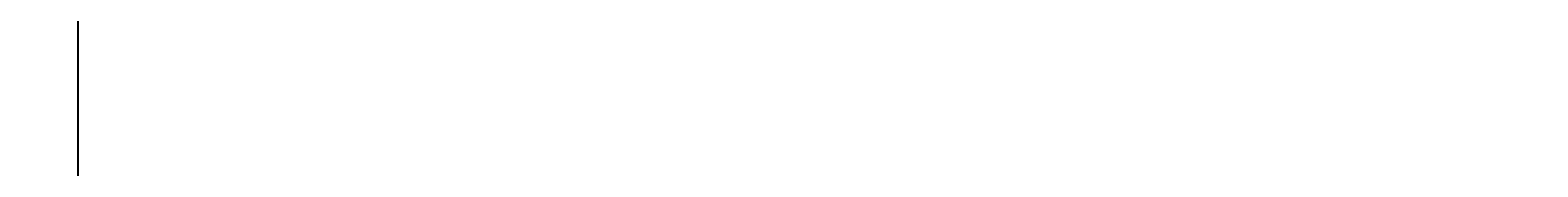
# Model space of a CAD drawing. Units: inches. Extents: x 35362 to 73946, y 43607 to 67532.
# Tile 103 of 134: x 50119 to 50761, y 49328 to 49386. Entities that reach past the tile are written whole.
import ezdxf

# ---------------------------------------------------------------- set-up
doc = ezdxf.new("R2010")
doc.units = ezdxf.units.IN
doc.header["$MEASUREMENT"] = 0
doc.layers.add('A-ANNO-DIMS', color=2, linetype='Continuous', lineweight=18)
doc.styles.get("Standard").update_dxf_attribs({"font": 'arial.ttf'})
doc.dimstyles.get("Standard").update_dxf_attribs({"dimtxt": 0.18, "dimasz": 0.18, "dimexe": 0.18, "dimexo": 0.0625, "dimgap": 0.09, "dimtad": 0, "dimtih": 1, "dimtoh": 1, "dimdec": 4, "dimzin": 0, "dimdsep": 46, "dimtxsty": 'Standard', "dimcen": 0.09, "dimadec": 0, "dimazin": 0, "dimtfac": 1, "dimtdec": 4, "dimtofl": 0, "dimtmove": 0, "dimatfit": 3, "dimfxl": 1, "dimtolj": 1, "dimtzin": 0, "dimarcsym": 0})

# ---------------------------------------------------------------- blocks, each defined once
blk = doc.blocks.new('*D11')
at = {"layer": 'A-ANNO-DIMS', "color": 0, "lineweight": -2, "transparency": 16777216}
for p, q in [((47978.66, 56028.77), (47978.66, 43606.68)), ((53109.76, 56028.77), (53109.76, 43606.68)), ((47978.84, 43606.86), (50543.87, 43606.86)), ((53109.58, 43606.86), (50544.55, 43606.86))]:
    blk.add_line(p, q, dxfattribs=at)
at = {"layer": 'A-ANNO-DIMS', "color": 0, "transparency": 16777216}
for points in [[(47978.84, 43606.89), (47978.84, 43606.83), (47978.66, 43606.86)], [(53109.58, 43606.89), (53109.58, 43606.83), (53109.76, 43606.86)]]:
    blk.add_solid(points, dxfattribs=at)
at = {"layer": 'Defpoints', "color": 0, "transparency": 16777216}
for p in [(47978.66, 56028.84), (53109.76, 56028.84), (53109.76, 43606.86)]:
    blk.add_point(p, dxfattribs=at)
at = {"layer": 'A-ANNO-DIMS', "color": 0, "transparency": 16777216, "insert": (50544.21, 43606.86), "char_height": 0.18, "attachment_point": 5}
blk.add_mtext('\\A1;5131', dxfattribs=at)
blk = doc.blocks.new('*D13')
at = {"layer": 'A-ANNO-DIMS', "color": 0, "lineweight": -2, "transparency": 16777216}
for p, q in [((48373.49, 51694.02), (48373.49, 43606.68)), ((51029.04, 51694.02), (51029.04, 43606.68)), ((48373.67, 43606.86), (49700.8, 43606.86)), ((51028.86, 43606.86), (49701.73, 43606.86))]:
    blk.add_line(p, q, dxfattribs=at)
at = {"layer": 'A-ANNO-DIMS', "color": 0, "transparency": 16777216}
for points in [[(48373.67, 43606.89), (48373.67, 43606.83), (48373.49, 43606.86)], [(51028.86, 43606.89), (51028.86, 43606.83), (51029.04, 43606.86)]]:
    blk.add_solid(points, dxfattribs=at)
at = {"layer": 'Defpoints', "color": 0, "transparency": 16777216}
for p in [(48373.49, 51694.09), (51029.04, 51694.09), (51029.04, 43606.86)]:
    blk.add_point(p, dxfattribs=at)
at = {"layer": 'A-ANNO-DIMS', "color": 0, "transparency": 16777216, "insert": (49701.27, 43606.86), "char_height": 0.18, "attachment_point": 5}
blk.add_mtext('\\A1;2655.6', dxfattribs=at)
blk = doc.blocks.new('*D17')
at = {"layer": 'A-ANNO-DIMS', "color": 0, "lineweight": -2, "transparency": 16777216}
for p, q in [((49923.31, 61293.22), (49923.31, 43606.68)), ((51913.93, 61293.22), (51913.93, 43606.68)), ((49923.49, 43606.86), (50918.16, 43606.86)), ((51913.75, 43606.86), (50919.07, 43606.86))]:
    blk.add_line(p, q, dxfattribs=at)
at = {"layer": 'A-ANNO-DIMS', "color": 0, "transparency": 16777216}
for points in [[(49923.49, 43606.89), (49923.49, 43606.83), (49923.31, 43606.86)], [(51913.75, 43606.89), (51913.75, 43606.83), (51913.93, 43606.86)]]:
    blk.add_solid(points, dxfattribs=at)
at = {"layer": 'Defpoints', "color": 0, "transparency": 16777216}
for p in [(49923.31, 61293.29), (51913.93, 61293.29), (51913.93, 43606.86)]:
    blk.add_point(p, dxfattribs=at)
at = {"layer": 'A-ANNO-DIMS', "color": 0, "transparency": 16777216, "insert": (50918.62, 43606.86), "char_height": 0.18, "attachment_point": 5}
blk.add_mtext('\\A1;1990.6', dxfattribs=at)
blk = doc.blocks.new('*D40')
at = {"layer": 'A-ANNO-DIMS', "color": 0, "lineweight": -2, "transparency": 16777216}
for p, q in [((56873.54, 53351.53), (35361.77, 53351.53)), ((35361.95, 53351.35), (35361.95, 51333.28)), ((35361.95, 49314.85), (35361.95, 51332.92)), ((51806.45, 49314.67), (35361.77, 49314.67))]:
    blk.add_line(p, q, dxfattribs=at)
at = {"layer": 'A-ANNO-DIMS', "color": 0, "transparency": 16777216}
for points in [[(35361.92, 53351.35), (35361.98, 53351.35), (35361.95, 53351.53)], [(35361.92, 49314.85), (35361.98, 49314.85), (35361.95, 49314.67)]]:
    blk.add_solid(points, dxfattribs=at)
at = {"layer": 'Defpoints', "color": 0, "transparency": 16777216}
for p in [(35361.95, 53351.53), (56873.6, 53351.53), (51806.52, 49314.67)]:
    blk.add_point(p, dxfattribs=at)
at = {"layer": 'A-ANNO-DIMS', "color": 0, "transparency": 16777216, "insert": (35361.95, 51333.1), "char_height": 0.18, "attachment_point": 5}
blk.add_mtext('\\A1;4036.9', dxfattribs=at)
blk = doc.blocks.new('*D67')
at = {"layer": 'A-ANNO-DIMS', "color": 0, "lineweight": -2, "transparency": 16777216}
for p, q in [((56873.54, 53351.53), (35361.77, 53351.53)), ((35361.95, 53351.35), (35361.95, 49400.89)), ((35361.95, 45450.07), (35361.95, 49400.53)), ((53793.58, 45449.89), (35361.77, 45449.89))]:
    blk.add_line(p, q, dxfattribs=at)
at = {"layer": 'A-ANNO-DIMS', "color": 0, "transparency": 16777216}
for points in [[(35361.92, 53351.35), (35361.98, 53351.35), (35361.95, 53351.53)], [(35361.92, 45450.07), (35361.98, 45450.07), (35361.95, 45449.89)]]:
    blk.add_solid(points, dxfattribs=at)
at = {"layer": 'Defpoints', "color": 0, "transparency": 16777216}
for p in [(35361.95, 53351.53), (56873.6, 53351.53), (53793.64, 45449.89)]:
    blk.add_point(p, dxfattribs=at)
at = {"layer": 'A-ANNO-DIMS', "color": 0, "transparency": 16777216, "insert": (35361.95, 49400.71), "char_height": 0.18, "attachment_point": 5}
blk.add_mtext('\\A1;7901.6', dxfattribs=at)
blk = doc.blocks.new('*D107')
at = {"layer": 'A-ANNO-DIMS', "color": 0, "lineweight": -2, "transparency": 16777216}
for p, q in [((50139.56, 59850.01), (50139.56, 43606.68)), ((51320.81, 59850.01), (51320.81, 43606.68)), ((50139.74, 43606.86), (50729.73, 43606.86)), ((51320.63, 43606.86), (50730.64, 43606.86))]:
    blk.add_line(p, q, dxfattribs=at)
at = {"layer": 'A-ANNO-DIMS', "color": 0, "transparency": 16777216}
for points in [[(50139.74, 43606.89), (50139.74, 43606.83), (50139.56, 43606.86)], [(51320.63, 43606.89), (51320.63, 43606.83), (51320.81, 43606.86)]]:
    blk.add_solid(points, dxfattribs=at)
at = {"layer": 'Defpoints', "color": 0, "transparency": 16777216}
for p in [(50139.56, 59850.08), (51320.81, 59850.08), (51320.81, 43606.86)]:
    blk.add_point(p, dxfattribs=at)
at = {"layer": 'A-ANNO-DIMS', "color": 0, "transparency": 16777216, "insert": (50730.19, 43606.86), "char_height": 0.18, "attachment_point": 5}
blk.add_mtext('\\A1;1181.3', dxfattribs=at)

msp = doc.modelspace()

# ---------------------------------------------------------------- dimensions: what is measured, and where the dimension line sits
at = {"layer": 'A-ANNO-DIMS'}
for base, p1, p2, override, picture, middle in [((51913.931, 43606.859), (49923.307, 61293.286), (51913.931, 61293.286), {"dimdec": 1, "dimlfac": 1, "dimrnd": 0, "dimzin": 0, "dimdsep": 46, "dimlunit": 2}, '*D17', (50918.619, 43606.859)), ((51320.8133, 43606.859), (50139.5627, 59850.0769), (51320.8133, 59850.0769), {"dimdec": 1, "dimlfac": 1, "dimrnd": 0, "dimzin": 0, "dimdsep": 46, "dimlunit": 2}, '*D107', (50730.188, 43606.859)), ((53109.76, 43606.859), (47978.665, 56028.836), (53109.76, 56028.836), {"dimdec": 0, "dimlfac": 1, "dimrnd": 0, "dimzin": 0, "dimdsep": 46, "dimlunit": 2}, '*D11', (50544.212, 43606.859)), ((51029.043, 43606.859), (48373.492, 51694.087), (51029.043, 51694.087), {"dimdec": 1, "dimlfac": 1, "dimrnd": 0, "dimzin": 0, "dimdsep": 46, "dimlunit": 2}, '*D13', (49701.267, 43606.859))]:
    dim = msp.add_linear_dim(base=base, p1=p1, p2=p2, dimstyle='Standard', override=override, dxfattribs=at)
    dim.commit()
    dim.dimension.update_dxf_attribs({"geometry": picture, "text_midpoint": middle})
for p1, picture, middle in [((51806.517, 49314.669), '*D40', (35361.949, 51333.099)), ((53793.638, 45449.894), '*D67', (35361.949, 49400.712))]:
    dim = msp.add_linear_dim(base=(35361.949, 53351.529), p1=p1, p2=(56873.602, 53351.529), angle=90, dimstyle='Standard', override={"dimdec": 1, "dimlfac": 1, "dimrnd": 0, "dimzin": 0, "dimdsep": 46, "dimlunit": 2}, dxfattribs=at)
    dim.commit()
    dim.dimension.update_dxf_attribs({"geometry": picture, "text_midpoint": middle})

doc.saveas('drawing.dxf')
